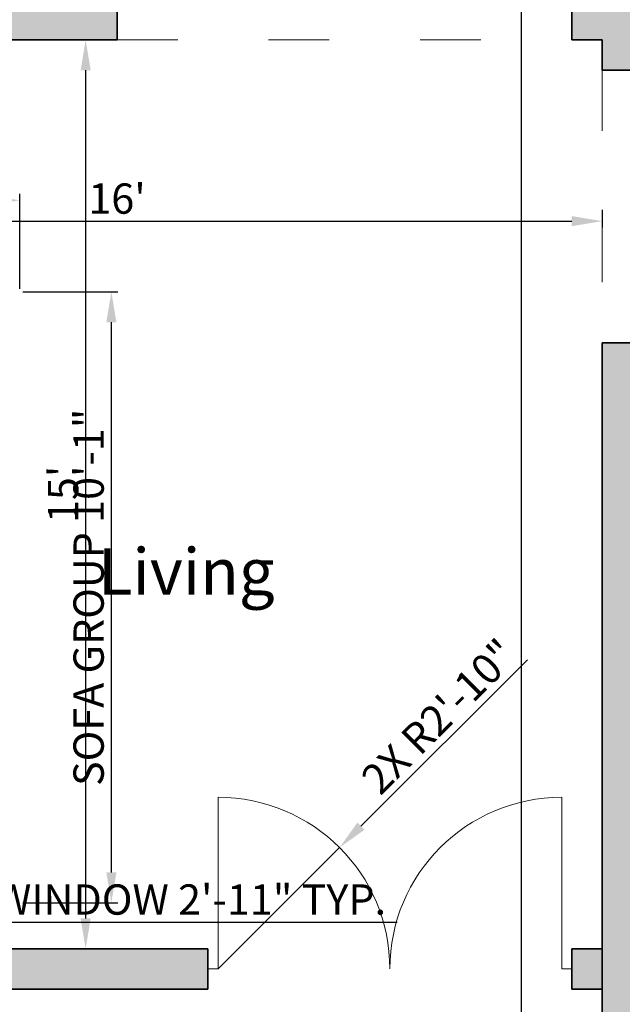
# Model space of a CAD drawing. Units: inches. Extents: x 2129 to 3258, y 1851 to 3021.
# Tile 3 of 10: x 2271 to 2390, y 1956 to 2151. Entities that reach past the tile are written whole.
import ezdxf

# ---------------------------------------------------------------- set-up
doc = ezdxf.new("R2010")
doc.units = ezdxf.units.IN
doc.linetypes.add('ACAD_ISO03W100', pattern=[30, 12, -18])
for name, color, linetype, lineweight in [('A-ANNO-DIMS', 2, 'Continuous', 18), ('A-AREA-IDEN', 7, 'Continuous', 20), ('A-DOOR', 4, 'Continuous', 18), ('A-WALL', 7, 'Continuous', 35), ('A-WALL-OVHD', 8, 'ACAD_ISO03W100', 18)]:
    doc.layers.add(name, color=color, linetype=linetype, lineweight=lineweight)
doc.layers.add('A-WALL-PATT', color=32, linetype='Continuous', lineweight=13, true_color=0xcd6928)
doc.styles.get("Standard").update_dxf_attribs({"font": 'arial.ttf'})
doc.dimstyles.new('ISO-25', dxfattribs={"dimtxt": 6, "dimasz": 6, "dimexe": 1.25, "dimexo": 0.625, "dimtad": 1, "dimdec": 1, "dimlunit": 3, "dimtxsty": 'Standard', "dimcen": 2.5, "dimclrd": 5, "dimclre": 5, "dimadec": 0, "dimazin": 0, "dimtfac": 1, "dimtdec": 1, "dimtmove": 0, "dimatfit": 3, "dimfxl": 1, "dimarcsym": 0})

# ---------------------------------------------------------------- blocks, each defined once
blk = doc.blocks.new('*D9')
at = {"layer": 'A-ANNO-DIMS', "color": 0, "lineweight": -2, "transparency": 16777216}
for p, q in [((2193.93, 2115.34), (2193.93, 2110.09)), ((2385.93, 2113.61), (2385.93, 2110.09)), ((2199.93, 2111.34), (2379.93, 2111.34))]:
    blk.add_line(p, q, dxfattribs=at)
at = {"layer": 'A-ANNO-DIMS', "color": 0, "transparency": 16777216}
for points in [[(2199.93, 2112.34), (2199.93, 2110.34), (2193.93, 2111.34)], [(2379.93, 2112.34), (2379.93, 2110.34), (2385.93, 2111.34)]]:
    blk.add_solid(points, dxfattribs=at)
at = {"layer": 'Defpoints', "color": 0, "transparency": 16777216}
for p in [(2193.93, 2115.96), (2385.93, 2114.23), (2385.93, 2111.34)]:
    blk.add_point(p, dxfattribs=at)
at = {"layer": 'A-ANNO-DIMS', "color": 0, "transparency": 16777216, "insert": (2289.93, 2115.03), "char_height": 6, "attachment_point": 5}
blk.add_mtext("16'", dxfattribs=at)
blk = doc.blocks.new('*D10')
at = {"layer": 'A-ANNO-DIMS', "color": 0, "lineweight": -2, "transparency": 16777216}
for p, q in [((2279.73, 2147.23), (2284.97, 2147.23)), ((2283.72, 2141.23), (2283.72, 1973.23)), ((2279.73, 1967.23), (2284.97, 1967.23))]:
    blk.add_line(p, q, dxfattribs=at)
at = {"layer": 'A-ANNO-DIMS', "color": 0, "transparency": 16777216}
for points in [[(2282.72, 2141.23), (2284.72, 2141.23), (2283.72, 2147.23)], [(2282.72, 1973.23), (2284.72, 1973.23), (2283.72, 1967.23)]]:
    blk.add_solid(points, dxfattribs=at)
at = {"layer": 'Defpoints', "color": 0, "transparency": 16777216}
for p in [(2279.11, 2147.23), (2279.11, 1967.23), (2283.72, 1967.23)]:
    blk.add_point(p, dxfattribs=at)
at = {"layer": 'A-ANNO-DIMS', "color": 0, "transparency": 16777216, "insert": (2280.03, 2057.23), "char_height": 6, "attachment_point": 5, "rotation": 90}
blk.add_mtext("15'", dxfattribs=at)
blk = doc.blocks.new('*D62')
at = {"layer": 'A-ANNO-DIMS', "color": 5, "lineweight": -2, "transparency": 16777216}
for p, q in [((2222.56, 1967.86), (2222.56, 1973.73)), ((2257.56, 1967.86), (2257.56, 1973.73)), ((2228.56, 1972.48), (2251.56, 1972.48)), ((2257.56, 1972.48), (2345.4, 1972.48))]:
    blk.add_line(p, q, dxfattribs=at)
at = {"layer": 'A-ANNO-DIMS', "color": 5, "transparency": 16777216}
for points in [[(2228.56, 1973.48), (2228.56, 1971.48), (2222.56, 1972.48)], [(2251.56, 1973.48), (2251.56, 1971.48), (2257.56, 1972.48)]]:
    blk.add_solid(points, dxfattribs=at)
at = {"layer": 'Defpoints', "color": 0, "transparency": 16777216}
for p in [(2257.56, 1972.48), (2222.56, 1967.23), (2257.56, 1967.23)]:
    blk.add_point(p, dxfattribs=at)
at = {"layer": 'A-ANNO-DIMS', "color": 0, "transparency": 16777216, "insert": (2304.48, 1976.21), "char_height": 6, "attachment_point": 5}
blk.add_mtext('WINDOW 2\'-11" TYP.', dxfattribs=at)
blk = doc.blocks.new('*D76')
at = {"layer": 'A-ANNO-DIMS', "color": 5, "lineweight": -2, "transparency": 16777216}
for p, q in [((2271.29, 2097.32), (2290.06, 2097.32)), ((2288.81, 1982.36), (2288.81, 2091.32)), ((2271.29, 1976.36), (2290.06, 1976.36))]:
    blk.add_line(p, q, dxfattribs=at)
at = {"layer": 'A-ANNO-DIMS', "color": 5, "transparency": 16777216}
for points in [[(2287.81, 2091.32), (2289.81, 2091.32), (2288.81, 2097.32)], [(2287.81, 1982.36), (2289.81, 1982.36), (2288.81, 1976.36)]]:
    blk.add_solid(points, dxfattribs=at)
at = {"layer": 'Defpoints', "color": 0, "transparency": 16777216}
for p in [(2270.67, 2097.32), (2288.81, 2097.32), (2270.67, 1976.36)]:
    blk.add_point(p, dxfattribs=at)
at = {"layer": 'A-ANNO-DIMS', "color": 0, "transparency": 16777216, "insert": (2285.08, 2036.84), "char_height": 6, "attachment_point": 5, "rotation": 90}
blk.add_mtext('SOFA GROUP 10\'-1"', dxfattribs=at)
blk = doc.blocks.new('*D77')
at = {"layer": 'A-ANNO-DIMS', "color": 5, "lineweight": -2, "transparency": 16777216}
for p, q in [((2202.74, 2097.95), (2202.74, 2116.72)), ((2270.67, 2097.95), (2270.67, 2116.72)), ((2264.67, 2115.47), (2208.74, 2115.47))]:
    blk.add_line(p, q, dxfattribs=at)
at = {"layer": 'A-ANNO-DIMS', "color": 5, "transparency": 16777216}
for points in [[(2208.74, 2116.47), (2208.74, 2114.47), (2202.74, 2115.47)], [(2264.67, 2116.47), (2264.67, 2114.47), (2270.67, 2115.47)]]:
    blk.add_solid(points, dxfattribs=at)
at = {"layer": 'Defpoints', "color": 0, "transparency": 16777216}
for p in [(2202.74, 2115.47), (2202.74, 2097.32), (2270.67, 2097.32)]:
    blk.add_point(p, dxfattribs=at)
at = {"layer": 'A-ANNO-DIMS', "color": 0, "transparency": 16777216, "insert": (2236.71, 2119.16), "char_height": 6, "attachment_point": 5}
blk.add_mtext('5\'-8"', dxfattribs=at)
blk = doc.blocks.new('*D91')
at = {"layer": 'A-ANNO-DIMS', "color": 5, "lineweight": -2, "transparency": 16777216}
for p, q in [((2369.93, 2314.61), (2369.93, 1851.23)), ((2429.93, 2314.61), (2429.93, 1851.23)), ((2375.93, 1852.48), (2423.93, 1852.48))]:
    blk.add_line(p, q, dxfattribs=at)
at = {"layer": 'A-ANNO-DIMS', "color": 5, "transparency": 16777216}
for points in [[(2375.93, 1853.48), (2375.93, 1851.48), (2369.93, 1852.48)], [(2423.93, 1853.48), (2423.93, 1851.48), (2429.93, 1852.48)]]:
    blk.add_solid(points, dxfattribs=at)
at = {"layer": 'Defpoints', "color": 0, "transparency": 16777216}
for p in [(2369.93, 2315.23), (2429.93, 2315.23), (2429.93, 1852.48)]:
    blk.add_point(p, dxfattribs=at)
at = {"layer": 'A-ANNO-DIMS', "color": 0, "transparency": 16777216, "insert": (2399.93, 1856.17), "char_height": 6, "attachment_point": 5}
blk.add_mtext('5\'-0"', dxfattribs=at)
blk = doc.blocks.new('*D138')
at = {"layer": 'A-ANNO-DIMS', "color": 5, "lineweight": -2, "transparency": 16777216}
for p, q in [((2371.16, 2024.47), (2338.21, 1991.52)), ((2309.93, 1963.23), (2333.97, 1987.28))]:
    blk.add_line(p, q, dxfattribs=at)
at = {"layer": 'A-ANNO-DIMS', "color": 5, "transparency": 16777216}
blk.add_solid([(2337.51, 1992.23), (2338.92, 1990.81), (2333.97, 1987.28)], dxfattribs=at)
at = {"layer": 'Defpoints', "color": 0, "transparency": 16777216}
for p in [(2333.97, 1987.28), (2309.93, 1963.23)]:
    blk.add_point(p, dxfattribs=at)
at = {"layer": 'A-ANNO-DIMS', "color": 0, "transparency": 16777216, "insert": (2354.2, 2012.72), "char_height": 6, "attachment_point": 5, "rotation": 44.9992}
blk.add_mtext('2X R2\'-10"', dxfattribs=at)

msp = doc.modelspace()

# ---------------------------------------------------------------- hatches: boundary and pattern name
at = {"layer": 'A-WALL-PATT'}
h = msp.add_hatch(color=256, dxfattribs=at)
h.dxf.hatch_style = 1
h.paths.add_polyline_path([(2393.39, 2407.23), (2185.93, 2407.23), (2185.93, 2394.06), (2193.93, 2394.06), (2193.93, 2399.23), (2361.93, 2399.23), (2361.93, 2355.23), (2361.93, 2347.23), (2361.93, 2258.25), (2369.93, 2258.25), (2369.93, 2307.23), (2429.93, 2307.23), (2429.93, 2303.23), (2437.93, 2303.23), (2437.93, 2327.23), (2429.93, 2327.23), (2429.93, 2315.23), (2369.93, 2315.23), (2369.93, 2399.23), (2393.39, 2399.23)])
h.paths.add_polyline_path([(2569.93, 2407.23), (2410.42, 2407.23), (2410.42, 2399.23), (2429.93, 2399.23), (2429.93, 2351.23), (2437.93, 2351.23), (2437.93, 2399.23), (2561.93, 2399.23), (2561.93, 2317.22), (2569.93, 2317.22)])
h.paths.add_polyline_path([(2569.93, 2282.22), (2561.93, 2282.22), (2561.93, 2243.23), (2437.93, 2243.23), (2437.93, 2249.23), (2429.93, 2249.23), (2429.93, 2235.23), (2561.93, 2235.23), (2561.93, 2155.23), (2379.93, 2155.23), (2379.93, 2147.23), (2385.93, 2147.23), (2385.93, 2141.23), (2393.93, 2141.23), (2393.93, 2147.23), (2469.93, 2147.23), (2469.93, 2111.23), (2477.93, 2111.23), (2477.93, 2147.23), (2561.93, 2147.23), (2561.93, 2129.53), (2569.93, 2129.53)])
h.paths.add_polyline_path([(2569.93, 2112.5), (2561.93, 2112.5), (2561.93, 2063.23), (2477.93, 2063.23), (2477.93, 2069.23), (2469.93, 2069.23), (2469.93, 2063.23), (2445.93, 2063.23), (2445.93, 2055.23), (2561.93, 2055.23), (2561.93, 1951.04), (2569.93, 1951.04)])
h.paths.add_polyline_path([(2569.93, 1916.04), (2561.93, 1916.04), (2561.93, 1887.23), (2393.93, 1887.23), (2393.93, 2055.23), (2399.93, 2055.23), (2399.93, 2063.23), (2393.93, 2063.23), (2393.93, 2087.23), (2385.93, 2087.23), (2385.93, 1887.23), (2385.93, 1879.23), (2569.93, 1879.23)])
h.paths.add_polyline_path([(2193.93, 2147.23), (2289.93, 2147.23), (2289.93, 2155.23), (2193.93, 2155.23), (2193.93, 2170.77), (2185.93, 2170.77), (2185.93, 2056.85), (2193.93, 2056.85)])
h.paths.add_polyline_path([(2193.93, 2021.85), (2185.93, 2021.85), (2185.93, 1959.23), (2222.56, 1959.23), (2222.56, 1967.23), (2193.93, 1967.23)])
h.paths.add_polyline_path([(2307.93, 1967.23), (2257.56, 1967.23), (2257.56, 1959.23), (2307.93, 1959.23)])
h.paths.add_polyline_path([(2255.61, 2368.18), (2321.09, 2368.18), (2321.09, 2384.66), (2255.61, 2384.66)], flags=25)
h.paths.add_polyline_path([(2282.89, 2032.34), (2325.27, 2032.34), (2325.27, 2051.27), (2282.89, 2051.27)], flags=9)
h.paths.add_polyline_path([(2404.09, 1945.18), (2463.36, 1945.18), (2463.36, 1961.66), (2404.09, 1961.66)], flags=25)
h.paths.add_polyline_path([(2494.41, 2286.84), (2553.68, 2286.84), (2553.68, 2303.32), (2494.41, 2303.32)], flags=9)
h.paths.add_polyline_path([(2389.71, 2321.98), (2411.09, 2321.98), (2411.09, 2338.47), (2389.71, 2338.47)], flags=25)
h.paths.add_polyline_path([(2219.41, 2162.82), (2258.18, 2162.82), (2258.18, 2179.3), (2219.41, 2179.3)], flags=9)
h.paths.add_polyline_path([(2249.68, 2306.23), (2298.12, 2306.23), (2298.12, 2323.98), (2249.68, 2323.98)], flags=25)
h = msp.add_hatch(color=256, dxfattribs=at)
h.dxf.hatch_style = 1
h.paths.add_polyline_path([(2193.93, 2288.35), (2185.93, 2288.35), (2185.93, 2205.77), (2193.93, 2205.77)])
h.paths.add_polyline_path([(2193.93, 2347.23), (2310.77, 2347.23), (2310.77, 2355.23), (2193.93, 2355.23), (2193.93, 2359.06), (2185.93, 2359.06), (2185.93, 2323.35), (2193.93, 2323.35)])
h.paths.add_polyline_path([(2314.44, 2244.01), (2314.44, 2257.94), (2302.07, 2257.94), (2302.07, 2244.01)], flags=9)
h.paths.add_polyline_path([(2255.61, 2368.18), (2321.09, 2368.18), (2321.09, 2384.66), (2255.61, 2384.66)], flags=9)
h.paths.add_polyline_path([(2282.89, 2032.34), (2325.27, 2032.34), (2325.27, 2051.27), (2282.89, 2051.27)], flags=9)
h.paths.add_polyline_path([(2404.09, 1945.18), (2463.36, 1945.18), (2463.36, 1961.66), (2404.09, 1961.66)], flags=9)
h.paths.add_polyline_path([(2494.41, 2286.84), (2553.68, 2286.84), (2553.68, 2303.32), (2494.41, 2303.32)], flags=9)
h.paths.add_polyline_path([(2389.71, 2321.98), (2411.09, 2321.98), (2411.09, 2338.47), (2389.71, 2338.47)], flags=9)
h.paths.add_polyline_path([(2219.41, 2162.82), (2258.18, 2162.82), (2258.18, 2179.3), (2219.41, 2179.3)], flags=9)
h.paths.add_polyline_path([(2249.68, 2306.23), (2298.12, 2306.23), (2298.12, 2323.98), (2249.68, 2323.98)], flags=9)
h = msp.add_hatch(color=256, dxfattribs=at)
h.dxf.hatch_style = 1
h.paths.add_polyline_path([(2385.93, 1967.23), (2379.93, 1967.23), (2379.93, 1959.23), (2385.93, 1959.23)])

# ---------------------------------------------------------------- linework, layer by layer
at = {"layer": 'A-DOOR'}
for p, q in [((2309.93, 1963.23), (2309.93, 1997.23)), ((2377.93, 1997.23), (2377.93, 1963.23)), ((2307.93, 1963.23), (2309.93, 1963.23)), ((2379.93, 1963.23), (2377.93, 1963.23))]:
    msp.add_line(p, q, dxfattribs=at)
for centre, start, end in [((2309.93, 1963.23), 360, 90), ((2377.93, 1963.23), 90, 180)]:
    msp.add_arc(centre, 34, start, end, dxfattribs=at)
at = {"layer": 'A-WALL'}
for p, q in [((2289.93, 2147.23), (2289.93, 2155.23)), ((2379.93, 2147.23), (2379.93, 2155.23)), ((2193.93, 2147.23), (2289.93, 2147.23)), ((2379.93, 2147.23), (2385.93, 2147.23)), ((2385.93, 2141.23), (2385.93, 2147.23)), ((2385.93, 2141.23), (2393.93, 2141.23)), ((2385.93, 1887.23), (2385.93, 2087.23)), ((2393.93, 2087.23), (2385.93, 2087.23)), ((2193.93, 1967.23), (2307.93, 1967.23)), ((2307.93, 1959.23), (2307.93, 1967.23)), ((2379.93, 1967.23), (2379.93, 1959.23)), ((2379.93, 1967.23), (2385.93, 1967.23)), ((2185.93, 1959.23), (2307.93, 1959.23)), ((2379.93, 1959.23), (2385.93, 1959.23))]:
    msp.add_line(p, q, dxfattribs=at)
at = {"layer": 'A-WALL-OVHD'}
for p, q in [((2289.93, 2147.23), (2379.93, 2147.23)), ((2385.93, 2141.23), (2385.93, 2087.23))]:
    msp.add_line(p, q, dxfattribs=at)

# ---------------------------------------------------------------- texts
at = {"layer": 'A-AREA-IDEN', "insert": (2286.17, 2046.54), "char_height": 9.1872, "attachment_point": 1}
msp.add_mtext_dynamic_manual_height_columns('{\\fArial|b1|i0|c0|p34;Living}', width=40.2574, gutter_width=14.35, heights=[9.95], dxfattribs=at)

# ---------------------------------------------------------------- dimensions: what is measured, and where the dimension line sits
at = {"layer": 'A-ANNO-DIMS'}
for base, p1, p2, override, picture, middle in [((2429.93, 1852.48), (2369.93, 2315.23), (2429.93, 2315.23), {"dimdec": 1, "dimlfac": 1, "dimrnd": 0, "dimzin": 1, "dimdsep": 46, "dimlunit": 4, "dimfrac": 2}, '*D91', (2399.93, 1856.17)), ((2385.93, 2111.34), (2193.93, 2115.96), (2385.93, 2114.23), {"dimclrd": 0, "dimclre": 0, "dimclrt": 0}, '*D9', (2289.93, 2115.03))]:
    dim = msp.add_linear_dim(base=base, p1=p1, p2=p2, dimstyle='ISO-25', override=override, dxfattribs=at)
    dim.commit()
    dim.dimension.update_dxf_attribs({"geometry": picture, "text_midpoint": middle})
for base, p1, p2, angle, override, picture, middle in [((2283.72, 1967.23), (2279.11, 2147.23), (2279.11, 1967.23), 90, {"dimclrd": 0, "dimclre": 0, "dimclrt": 0}, '*D10', (2280.03, 2057.23)), ((2202.74, 2115.47), (2270.67, 2097.32), (2202.74, 2097.32), 180, {"dimdec": 1, "dimlfac": 1, "dimrnd": 0, "dimzin": 1, "dimdsep": 46, "dimlunit": 4, "dimfrac": 2}, '*D77', (2236.71, 2119.16))]:
    dim = msp.add_linear_dim(base=base, p1=p1, p2=p2, angle=angle, dimstyle='ISO-25', override=override, dxfattribs=at)
    dim.commit()
    dim.dimension.update_dxf_attribs({"geometry": picture, "text_midpoint": middle})
dim = msp.add_linear_dim(base=(2288.81, 2097.32), p1=(2270.67, 1976.36), p2=(2270.67, 2097.32), angle=90, text='SOFA GROUP <>', dimstyle='ISO-25', override={"dimdec": 1, "dimlfac": 1, "dimrnd": 0, "dimzin": 1, "dimdsep": 46, "dimlunit": 4, "dimfrac": 2}, dxfattribs=at)
dim.commit()
dim.dimension.update_dxf_attribs({"geometry": '*D76', "text_midpoint": (2285.08, 2036.84)})
dim = msp.add_radius_dim(center=(2309.93, 1963.23), mpoint=(2333.97, 1987.28), text='2X <>', dimstyle='ISO-25', override={"dimdec": 1, "dimlfac": 1, "dimrnd": 0, "dimzin": 1, "dimdsep": 46, "dimlunit": 4, "dimfrac": 2}, dxfattribs=at)
dim.commit()
dim.dimension.update_dxf_attribs({"geometry": '*D138', "text_midpoint": (2354.2, 2012.72)})
dim = msp.add_linear_dim(base=(2257.56, 1972.48), p1=(2222.56, 1967.23), p2=(2257.56, 1967.23), text='WINDOW <> TYP.', dimstyle='ISO-25', override={"dimdec": 1, "dimlfac": 1, "dimrnd": 0, "dimzin": 1, "dimdsep": 46, "dimlunit": 4, "dimfrac": 2}, dxfattribs=at)
dim.commit()
dim.dimension.update_dxf_attribs({"geometry": '*D62', "text_midpoint": (2304.48, 1976.21)})

doc.saveas('drawing.dxf')
